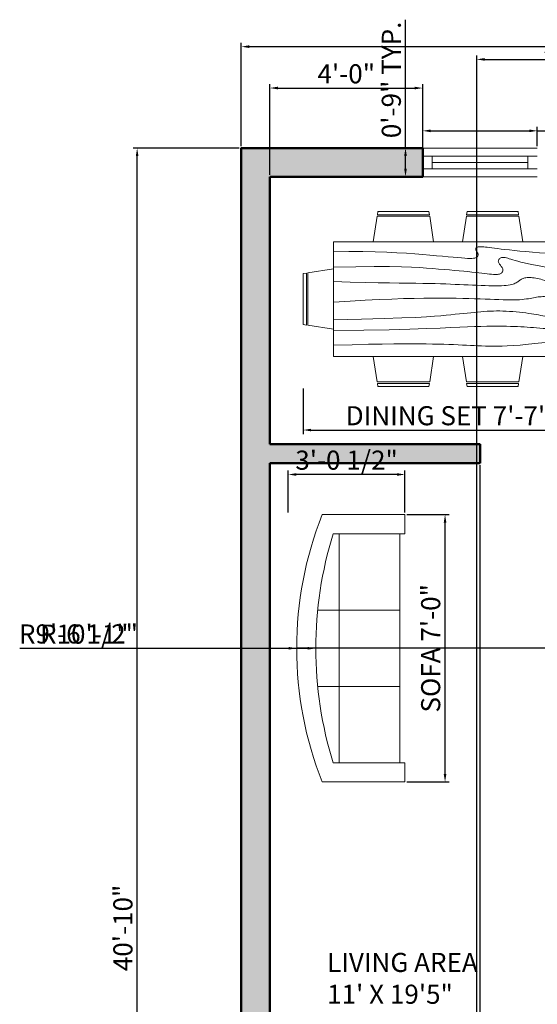
# Model space of a CAD drawing. Units: inches. Extents: x 2247 to 2697, y 1573 to 2133.
# Tile 2 of 4: x 2247 to 2409, y 1823 to 2133. Entities that reach past the tile are written whole.
import ezdxf

# ---------------------------------------------------------------- set-up
doc = ezdxf.new("R2010")
doc.units = ezdxf.units.IN
for name, color, linetype, lineweight in [('A-ANNO-DIMS', 2, 'Continuous', 18), ('A-AREA-IDEN', 7, 'Continuous', 25), ('A-FURN', 8, 'Continuous', 18), ('A-GLAZ', 4, 'Continuous', 18), ('A-WALL', 7, 'Continuous', 50)]:
    doc.layers.add(name, color=color, linetype=linetype, lineweight=lineweight)
doc.layers.add('A-WALL-PATT', color=67, linetype='Continuous', lineweight=13, true_color=0x727430)
doc.styles.get("Standard").update_dxf_attribs({"font": 'arial.ttf'})
doc.dimstyles.new('ISO-25', dxfattribs={"dimtxt": 6, "dimasz": 2.5, "dimexe": 1.25, "dimexo": 0.625, "dimtad": 1, "dimlunit": 3, "dimtxsty": 'Standard', "dimcen": 2.5, "dimadec": 0, "dimazin": 0, "dimtfac": 1, "dimtmove": 0, "dimatfit": 3, "dimfxl": 1, "dimarcsym": 0})

# ---------------------------------------------------------------- blocks, each defined once
blk = doc.blocks.new('*D1')
at = {"layer": 'A-ANNO-DIMS', "color": 0, "lineweight": -2, "transparency": 16777216}
for p, q in [((2316.09, 2092.98), (2316.09, 2125.46)), ((2617.09, 2092.98), (2617.09, 2125.46)), ((2318.59, 2124.21), (2614.59, 2124.21))]:
    blk.add_line(p, q, dxfattribs=at)
at = {"layer": 'A-ANNO-DIMS', "color": 0, "transparency": 16777216}
for points in [[(2318.59, 2124.63), (2318.59, 2123.79), (2316.09, 2124.21)], [(2614.59, 2124.63), (2614.59, 2123.79), (2617.09, 2124.21)]]:
    blk.add_solid(points, dxfattribs=at)
at = {"layer": 'Defpoints', "color": 0, "transparency": 16777216}
for p in [(2617.09, 2124.21), (2316.09, 2092.36), (2617.09, 2092.36)]:
    blk.add_point(p, dxfattribs=at)
at = {"layer": 'A-ANNO-DIMS', "color": 0, "transparency": 16777216, "insert": (2466.59, 2127.9), "char_height": 6, "attachment_point": 5}
blk.add_mtext('25\'-1"', dxfattribs=at)
blk = doc.blocks.new('*D3')
at = {"layer": 'A-ANNO-DIMS', "color": 0, "lineweight": -2, "transparency": 16777216}
for p, q in [((2315.47, 2092.36), (2282.14, 2092.36)), ((2283.39, 1604.86), (2283.39, 2089.86)), ((2315.47, 1602.36), (2282.14, 1602.36))]:
    blk.add_line(p, q, dxfattribs=at)
at = {"layer": 'A-ANNO-DIMS', "color": 0, "transparency": 16777216}
for points in [[(2282.98, 2089.86), (2283.81, 2089.86), (2283.39, 2092.36)], [(2282.98, 1604.86), (2283.81, 1604.86), (2283.39, 1602.36)]]:
    blk.add_solid(points, dxfattribs=at)
at = {"layer": 'Defpoints', "color": 0, "transparency": 16777216}
for p in [(2283.39, 2092.36), (2316.09, 2092.36), (2316.09, 1602.36)]:
    blk.add_point(p, dxfattribs=at)
at = {"layer": 'A-ANNO-DIMS', "color": 0, "transparency": 16777216, "insert": (2279.7, 1847.36), "char_height": 6, "attachment_point": 5, "rotation": 90}
blk.add_mtext('40\'-10"', dxfattribs=at)
blk = doc.blocks.new('Sofa - Roundback 7 ft.')
for p, q in [((-12.00002, -32.4421), (-12.00003, -6.5971)), ((11.99997, -32.4421), (11.99998, -6.5971)), ((-36.000027, -34), (-36.000027, -11.4696)), ((35.99998, -34), (35.99998, -11.4696)), ((-35.999844, -13.3819), (35.9998, -13.3819)), ((-36.000027, -32.4421), (35.99998, -32.4421))]:
    blk.add_line(p, q)
for points in [[(-36.000027, -34), (-42.000027, -34), (-42.000027, -8)], [(41.99998, -8), (41.99998, -34), (35.99998, -34)]]:
    blk.add_lwpolyline(points)
for centre, radius, start, end in [((0, -114.25), 114.25, 68.43141, 111.5686), ((-0.00001, -127.1968), 121.1968, 72.72033, 107.2797)]:
    blk.add_arc(centre, radius, start, end)
blk = doc.blocks.new('Dining Set - 36 x 72 in.')
for p, q in [((-22.2343, 26.00059), (-23.4847, 17.99762)), ((-22.2304, 26), (-5.7608, 26)), ((-22, 27.5), (-22.1562, 26.50042)), ((-5.8416, 26.5), (-22.1534, 26.5)), ((-22, 27.5), (-6, 27.5)), ((-5.8437, 26.49966), (-6, 27.5)), ((-4.5152, 17.99762), (-5.7655, 25.99926)), ((5.7657, 26.00059), (4.5153, 17.99762)), ((5.7696, 26), (22.2392, 26)), ((6, 27.5), (5.8438, 26.50042)), ((22.1584, 26.5), (5.8466, 26.5)), ((6, 27.5), (22, 27.5)), ((22.1563, 26.49966), (22, 27.5)), ((23.4848, 17.99762), (22.2345, 25.99926)), ((36, 18), (-36, 18)), ((-36, 18), (-36, -18)), ((36, -18), (36, 18)), ((-44.0006, 8.23428), (-35.9976, 9.48474)), ((44.0006, 8.23428), (35.9976, 9.48474)), ((-45.5, 8), (-44.5004, 8.15617)), ((-45.5, 8), (-45.5, -8)), ((-44.5, -8.15843), (-44.5, 8.15338)), ((-44, 8.23041), (-44, -8.23915)), ((44, 8.23041), (44, -8.23915)), ((44.5, -8.15843), (44.5, 8.15338)), ((45.5, 8), (44.5005, 8.15617)), ((45.5, 8), (45.5, -8)), ((-44.4997, -8.15631), (-45.5, -8)), ((-35.9976, -9.48476), (-43.9993, -8.2345)), ((35.9976, -9.48476), (43.9993, -8.2345)), ((44.4997, -8.15631), (45.5, -8)), ((-36, -18), (36, -18)), ((-22.2343, -26.0006), (-23.4847, -17.99762)), ((-4.5152, -17.99762), (-5.7655, -25.99928)), ((5.7657, -26.0006), (4.5153, -17.99762)), ((23.4848, -17.99762), (22.2345, -25.99928)), ((-22.2304, -26), (-5.7608, -26)), ((-22, -27.5), (-22.1562, -26.50044)), ((-5.8416, -26.5), (-22.1534, -26.5)), ((-22, -27.5), (-6, -27.5)), ((-5.8437, -26.49967), (-6, -27.5)), ((5.7696, -26), (22.2392, -26)), ((6, -27.5), (5.8438, -26.50044)), ((22.1584, -26.5), (5.8466, -26.5)), ((6, -27.5), (22, -27.5)), ((22.1563, -26.49967), (22, -27.5))]:
    blk.add_line(p, q)
for points in [[(-36, 15), (-31.1772, 14.97754), (-26.8079, 14.91406), (-22.8538, 14.81543), (-19.276, 14.6875), (-16.0362, 14.53613), (-13.0957, 14.36718), (-10.4159, 14.18652), (-7.9583, 14), (-5.6904, 13.81315), (-3.6035, 13.63021), (-1.6954, 13.45508), (0.0365, 13.29166), (1.5945, 13.14388), (2.9811, 13.01562), (4.1988, 12.9108), (5.25, 12.83333), (6.1393, 12.78613), (6.8802, 12.76823), (7.4883, 12.77767), (7.9792, 12.8125), (8.3685, 12.87077), (8.6719, 12.95052), (8.9049, 13.0498), (9.0833, 13.16666), (9.2205, 13.29899), (9.3216, 13.44401), (9.3895, 13.59879), (9.4271, 13.76041), (9.4373, 13.92594), (9.4232, 14.09245), (9.3875, 14.257), (9.3333, 14.41666), (9.2638, 14.56917), (9.1836, 14.71484), (9.0975, 14.85465), (9.0104, 14.98958), (8.9272, 15.1206), (8.8529, 15.2487), (8.7922, 15.37483), (8.75, 15.5), (8.7305, 15.62467), (8.7344, 15.74739), (8.7617, 15.86621), (8.8125, 15.97916), (8.8867, 16.08431), (8.9844, 16.17968), (9.1055, 16.26334), (9.25, 16.33333), (9.4189, 16.38802), (9.6172, 16.42708), (9.8506, 16.45052), (10.125, 16.45833), (10.4463, 16.45052), (10.8203, 16.42708), (11.2529, 16.38802), (11.75, 16.33333), (12.3184, 16.26318), (12.9694, 16.17838), (13.7151, 16.07991), (14.5677, 15.96875), (15.5395, 15.84586), (16.6426, 15.71224), (17.8893, 15.56884), (19.2917, 15.41666), (20.859, 15.25667), (22.5879, 15.08984), (24.4721, 14.91715), (26.5052, 14.73958), (28.6809, 14.5581), (30.9929, 14.3737), (33.4347, 14.18733), (36, 14)], [(-36, 10), (-28.9766, 10.14274), (-23.1725, 10.20442), (-18.4241, 10.19775), (-14.5677, 10.13541), (-11.4399, 10.03011), (-8.877, 9.89453), (-6.7154, 9.74137), (-4.7917, 9.58333), (-2.9698, 9.43082), (-1.2246, 9.28515), (0.4415, 9.14534), (2.026, 9.01041), (3.5266, 8.87939), (4.9408, 8.7513), (6.266, 8.62516), (7.5, 8.5), (8.6411, 8.37549), (9.6914, 8.2539), (10.6538, 8.13818), (11.5312, 8.03125), (12.3267, 7.93603), (13.043, 7.85547), (13.6831, 7.79248), (14.25, 7.75), (14.7471, 7.7303), (15.1797, 7.73307), (15.5537, 7.75732), (15.875, 7.80208), (16.1494, 7.86637), (16.3828, 7.94922), (16.5811, 8.04964), (16.75, 8.16666), (16.8944, 8.29915), (17.0143, 8.44531), (17.1089, 8.60319), (17.1771, 8.77083), (17.218, 8.94629), (17.2305, 9.1276), (17.2137, 9.31282), (17.1667, 9.5), (17.0895, 9.6875), (16.987, 9.875), (16.8649, 10.0625), (16.7292, 10.25), (16.5856, 10.4375), (16.4401, 10.625), (16.2985, 10.8125), (16.1667, 11), (16.05, 11.18733), (15.9518, 11.3737), (15.8752, 11.5581), (15.8229, 11.73958), (15.798, 11.91715), (15.8034, 12.08984), (15.842, 12.25667), (15.9167, 12.41666), (16.0295, 12.56836), (16.1784, 12.70833), (16.3605, 12.83268), (16.5729, 12.9375), (16.8127, 13.01888), (17.0768, 13.07291), (17.3625, 13.0957), (17.6667, 13.08333), (17.9894, 13.03312), (18.3418, 12.94726), (18.7382, 12.82918), (19.1927, 12.68229), (19.7195, 12.51001), (20.3327, 12.31575), (21.0465, 12.10294), (21.875, 11.875), (22.8357, 11.63354), (23.959, 11.37304), (25.2786, 11.08618), (26.8282, 10.76562), (28.6414, 10.40405), (30.752, 9.99414), (33.1936, 9.52856), (36, 9)], [(-36, 5.5), (-30.7157, 5.3348), (-26.069, 5.20963), (-21.9946, 5.11767), (-18.4271, 5.05208), (-15.3009, 5.00602), (-12.5508, 4.97265), (-10.1112, 4.94515), (-7.9167, 4.91666), (-5.909, 4.88167), (-4.0586, 4.83984), (-2.3429, 4.79215), (-0.7396, 4.73958), (0.7739, 4.6831), (2.22, 4.6237), (3.6213, 4.56233), (5, 4.5), (6.373, 4.43782), (7.7344, 4.3776), (9.0723, 4.32129), (10.375, 4.27083), (11.6309, 4.22819), (12.8281, 4.19531), (13.9551, 4.17415), (15, 4.16666), (15.954, 4.17448), (16.819, 4.19791), (17.6001, 4.23698), (18.3021, 4.29166), (18.9299, 4.36198), (19.4883, 4.44791), (19.9823, 4.54948), (20.4167, 4.66666), (20.7969, 4.79899), (21.1302, 4.94401), (21.4245, 5.09879), (21.6875, 5.26041), (21.9271, 5.42594), (22.1511, 5.59245), (22.3672, 5.757), (22.5834, 5.91666), (22.8065, 6.06868), (23.0404, 6.21093), (23.2879, 6.34147), (23.5521, 6.45833), (23.8358, 6.55957), (24.142, 6.64323), (24.4735, 6.70735), (24.8334, 6.75), (25.2235, 6.76969), (25.642, 6.76692), (26.0858, 6.74267), (26.5521, 6.69791), (27.0379, 6.63362), (27.5404, 6.55078), (28.0565, 6.45036), (28.5834, 6.33333), (29.1242, 6.19987), (29.7071, 6.04687), (30.3661, 5.87044), (31.1354, 5.66666), (32.0493, 5.43164), (33.142, 5.16146), (34.4475, 4.85221), (36, 4.5)], [(-36, -1), (-30.7915, -0.6591), (-26.0195, -0.38216), (-21.6519, -0.16284), (-17.6563, 0.00521), (-14.0005, 0.12833), (-10.6523, 0.21289), (-7.5796, 0.26522), (-4.75, 0.29166), (-2.134, 0.29793), (0.2878, 0.28711), (2.5317, 0.26163), (4.6146, 0.22396), (6.5529, 0.17651), (8.3633, 0.12174), (10.0623, 0.06209), (11.6667, 0), (13.1899, -0.06201), (14.6341, -0.1211), (15.9982, -0.17432), (17.2813, -0.21875), (18.4823, -0.25147), (19.6003, -0.26953), (20.6343, -0.27002), (21.5834, -0.25), (22.4481, -0.20768), (23.2357, -0.14584), (23.9549, -0.06836), (24.6146, 0.02083), (25.2235, 0.11784), (25.7904, 0.21875), (26.3241, 0.31966), (26.8334, 0.41666), (27.3265, 0.50618), (27.8099, 0.58593), (28.2894, 0.65397), (28.7709, 0.70833), (29.2601, 0.74707), (29.763, 0.76823), (30.2855, 0.76985), (30.8334, 0.75), (31.4088, 0.70784), (31.9994, 0.64713), (32.589, 0.57275), (33.1615, 0.48958), (33.7008, 0.4025), (34.1908, 0.3164), (34.6153, 0.23616), (34.9584, 0.16666), (35.2099, 0.11165), (35.3848, 0.07031), (35.504, 0.04069), (35.5886, 0.02083), (35.6594, 0.00879), (35.7377, 0.0026), (35.8442, 0.00032), (36, 0)], [(-36, -6.5), (-27.1843, -6.31267), (-20.084, -6.1263), (-14.469, -5.9419), (-10.1094, -5.76042), (-6.7752, -5.58285), (-4.2363, -5.41016), (-2.2629, -5.24333), (-0.625, -5.08334), (0.8708, -4.93099), (2.2715, -4.78646), (3.5872, -4.64974), (4.8281, -4.52084), (6.0046, -4.39974), (7.127, -4.28646), (8.2053, -4.18099), (9.25, -4.08334), (10.2705, -3.99382), (11.2734, -3.91407), (12.2647, -3.84603), (13.25, -3.79167), (14.2354, -3.75293), (15.2266, -3.73177), (16.2295, -3.73015), (17.25, -3.75), (18.2912, -3.79248), (19.3451, -3.85547), (20.4009, -3.93604), (21.4479, -4.03125), (22.4754, -4.13819), (23.4727, -4.25391), (24.4289, -4.37549), (25.3334, -4.5), (26.1785, -4.62492), (26.9694, -4.74935), (27.7145, -4.87281), (28.4219, -4.99479), (29.1, -5.11483), (29.7572, -5.23242), (30.4016, -5.34709), (31.0417, -5.45834), (31.6837, -5.56437), (32.3262, -5.65821), (32.9658, -5.73153), (33.599, -5.77604), (34.2224, -5.78345), (34.8327, -5.74545), (35.4264, -5.65373), (36, -5.5)], [(-36, -10), (-26.4022, -9.81299), (-18.4675, -9.62891), (-11.9839, -9.45069), (-6.7396, -9.28125), (-2.5226, -9.12354), (0.8789, -8.98047), (3.6769, -8.85498), (6.0833, -8.75), (8.2767, -8.66765), (10.3021, -8.60677), (12.1712, -8.56543), (13.8958, -8.54167), (15.4876, -8.53353), (16.9583, -8.53907), (18.3197, -8.55632), (19.5834, -8.58334), (20.7616, -8.61841), (21.8685, -8.66081), (22.9188, -8.71004), (23.9271, -8.76563), (24.9081, -8.82707), (25.8763, -8.89388), (26.8465, -8.96558), (27.8334, -9.04167), (28.8474, -9.12118), (29.8828, -9.20117), (30.93, -9.27824), (31.9792, -9.34896), (33.0205, -9.40991), (34.0443, -9.45768), (35.0407, -9.48885), (36, -9.5)], [(-36, -14.5), (-30.0881, -14.33513), (-25.0332, -14.21224), (-20.7312, -14.12647), (-17.0781, -14.07292), (-13.97, -14.04671), (-11.3027, -14.04297), (-8.9724, -14.05681), (-6.875, -14.08334), (-4.9224, -14.11833), (-3.0905, -14.16016), (-1.3709, -14.20785), (0.2448, -14.26042), (1.7647, -14.3169), (3.1973, -14.3763), (4.5507, -14.43767), (5.8333, -14.5), (7.0554, -14.5621), (8.235, -14.62175), (9.3922, -14.67652), (10.5469, -14.72396), (11.7192, -14.76164), (12.929, -14.78711), (14.1965, -14.79794), (15.5417, -14.79167), (16.9933, -14.76424), (18.6152, -14.70508), (20.4804, -14.60197), (22.6615, -14.44271), (25.2312, -14.21509), (28.2624, -13.9069), (31.8277, -13.50594), (36, -13)]]:
    blk.add_lwpolyline(points)
blk = doc.blocks.new('WIN-36IN')
for p, q in [((0, 9), (36, 9)), ((0, 6.5), (36, 6.5)), ((3, 2.5), (3, 6.5)), ((33, 2.5), (33, 6.5)), ((3, 4.5), (33, 4.5)), ((0, 2.5), (36, 2.5)), ((0, 0), (36, 0))]:
    blk.add_line(p, q)
blk = doc.blocks.new('*D13')
at = {"layer": 'A-ANNO-DIMS', "color": 0, "lineweight": -2, "transparency": 16777216}
for p, q in [((2373.09, 2092.98), (2373.09, 2099.01)), ((2375.59, 2097.76), (2406.59, 2097.76)), ((2409.09, 2092.98), (2409.09, 2099.01)), ((2409.09, 2097.76), (2488.77, 2097.76))]:
    blk.add_line(p, q, dxfattribs=at)
at = {"layer": 'A-ANNO-DIMS', "color": 0, "transparency": 16777216}
for points in [[(2375.59, 2098.18), (2375.59, 2097.34), (2373.09, 2097.76)], [(2406.59, 2098.18), (2406.59, 2097.34), (2409.09, 2097.76)]]:
    blk.add_solid(points, dxfattribs=at)
at = {"layer": 'Defpoints', "color": 0, "transparency": 16777216}
for p in [(2409.09, 2097.76), (2373.09, 2092.36), (2409.09, 2092.36)]:
    blk.add_point(p, dxfattribs=at)
at = {"layer": 'A-ANNO-DIMS', "color": 0, "transparency": 16777216, "insert": (2450.18, 2101.49), "char_height": 6, "attachment_point": 5}
blk.add_mtext('WINDOW 3\'-0" TYP.', dxfattribs=at)
blk = doc.blocks.new('*D14')
at = {"layer": 'A-ANNO-DIMS', "color": 0, "lineweight": -2, "transparency": 16777216}
for p, q in [((2367.69, 2092.36), (2367.69, 2132.68)), ((2372.47, 2092.36), (2366.44, 2092.36)), ((2367.69, 2085.86), (2367.69, 2089.86)), ((2372.47, 2083.36), (2366.44, 2083.36))]:
    blk.add_line(p, q, dxfattribs=at)
at = {"layer": 'A-ANNO-DIMS', "color": 0, "transparency": 16777216}
for points in [[(2367.28, 2089.86), (2368.11, 2089.86), (2367.69, 2092.36)], [(2367.28, 2085.86), (2368.11, 2085.86), (2367.69, 2083.36)]]:
    blk.add_solid(points, dxfattribs=at)
at = {"layer": 'Defpoints', "color": 0, "transparency": 16777216}
for p in [(2367.69, 2092.36), (2373.09, 2092.36), (2373.09, 2083.36)]:
    blk.add_point(p, dxfattribs=at)
at = {"layer": 'A-ANNO-DIMS', "color": 0, "transparency": 16777216, "insert": (2364.01, 2113.77), "char_height": 6, "attachment_point": 5, "rotation": 90}
blk.add_mtext('0\'-9" TYP.', dxfattribs=at)
blk = doc.blocks.new('*D19')
at = {"layer": 'A-ANNO-DIMS', "color": 0, "lineweight": -2, "transparency": 16777216}
for p, q in [((2368.14, 1977.2), (2381.36, 1977.2)), ((2380.11, 1895.7), (2380.11, 1974.7)), ((2368.14, 1893.2), (2381.36, 1893.2))]:
    blk.add_line(p, q, dxfattribs=at)
at = {"layer": 'A-ANNO-DIMS', "color": 0, "transparency": 16777216}
for points in [[(2379.7, 1974.7), (2380.53, 1974.7), (2380.11, 1977.2)], [(2379.7, 1895.7), (2380.53, 1895.7), (2380.11, 1893.2)]]:
    blk.add_solid(points, dxfattribs=at)
at = {"layer": 'Defpoints', "color": 0, "transparency": 16777216}
for p in [(2367.51, 1977.2), (2380.11, 1977.2), (2367.51, 1893.2)]:
    blk.add_point(p, dxfattribs=at)
at = {"layer": 'A-ANNO-DIMS', "color": 0, "transparency": 16777216, "insert": (2376.38, 1935.2), "char_height": 6, "attachment_point": 5, "rotation": 90}
blk.add_mtext('SOFA 7\'-0"', dxfattribs=at)
blk = doc.blocks.new('*D20')
at = {"layer": 'A-ANNO-DIMS', "color": 0, "lineweight": -2, "transparency": 16777216}
for p, q in [((2330.85, 1977.83), (2330.85, 1991.05)), ((2365.01, 1989.8), (2333.35, 1989.8)), ((2367.51, 1977.83), (2367.51, 1991.05))]:
    blk.add_line(p, q, dxfattribs=at)
at = {"layer": 'A-ANNO-DIMS', "color": 0, "transparency": 16777216}
for points in [[(2333.35, 1990.22), (2333.35, 1989.39), (2330.85, 1989.8)], [(2365.01, 1990.22), (2365.01, 1989.39), (2367.51, 1989.8)]]:
    blk.add_solid(points, dxfattribs=at)
at = {"layer": 'Defpoints', "color": 0, "transparency": 16777216}
for p in [(2330.85, 1989.8), (2330.85, 1977.2), (2367.51, 1977.2)]:
    blk.add_point(p, dxfattribs=at)
at = {"layer": 'A-ANNO-DIMS', "color": 0, "transparency": 16777216, "insert": (2349.18, 1993.53), "char_height": 6, "attachment_point": 5}
blk.add_mtext('3\'-0 1/2"', dxfattribs=at)
blk = doc.blocks.new('*D21')
at = {"layer": 'A-ANNO-DIMS', "color": 0, "lineweight": -2, "transparency": 16777216}
for p, q in [((2335.55, 2016.79), (2335.55, 2002.52)), ((2426.55, 2016.79), (2426.55, 2002.52)), ((2338.05, 2003.77), (2424.05, 2003.77))]:
    blk.add_line(p, q, dxfattribs=at)
at = {"layer": 'A-ANNO-DIMS', "color": 0, "transparency": 16777216}
for points in [[(2338.05, 2004.18), (2338.05, 2003.35), (2335.55, 2003.77)], [(2424.05, 2004.18), (2424.05, 2003.35), (2426.55, 2003.77)]]:
    blk.add_solid(points, dxfattribs=at)
at = {"layer": 'Defpoints', "color": 0, "transparency": 16777216}
for p in [(2335.55, 2017.42), (2426.55, 2017.42), (2426.55, 2003.77)]:
    blk.add_point(p, dxfattribs=at)
at = {"layer": 'A-ANNO-DIMS', "color": 0, "transparency": 16777216, "insert": (2381.05, 2007.49), "char_height": 6, "attachment_point": 5}
blk.add_mtext('DINING SET 7\'-7"', dxfattribs=at)
blk = doc.blocks.new('*D23')
at = {"layer": 'A-ANNO-DIMS', "color": 0, "lineweight": -2, "transparency": 16777216}
for p, q in [((2325.09, 2083.98), (2325.09, 2112.46)), ((2327.59, 2111.21), (2370.59, 2111.21)), ((2373.09, 2083.98), (2373.09, 2112.46))]:
    blk.add_line(p, q, dxfattribs=at)
at = {"layer": 'A-ANNO-DIMS', "color": 0, "transparency": 16777216}
for points in [[(2327.59, 2111.63), (2327.59, 2110.79), (2325.09, 2111.21)], [(2370.59, 2111.63), (2370.59, 2110.79), (2373.09, 2111.21)]]:
    blk.add_solid(points, dxfattribs=at)
at = {"layer": 'Defpoints', "color": 0, "transparency": 16777216}
for p in [(2373.09, 2111.21), (2325.09, 2083.36), (2373.09, 2083.36)]:
    blk.add_point(p, dxfattribs=at)
at = {"layer": 'A-ANNO-DIMS', "color": 0, "transparency": 16777216, "insert": (2349.09, 2114.9), "char_height": 6, "attachment_point": 5}
blk.add_mtext('4\'-0"', dxfattribs=at)
blk = doc.blocks.new('*D38')
at = {"layer": 'A-ANNO-DIMS', "color": 0, "lineweight": -2, "transparency": 16777216}
for p, q in [((2390.09, 1693.98), (2390.09, 2121.46)), ((2392.59, 2120.21), (2447.59, 2120.21)), ((2450.09, 1693.98), (2450.09, 2121.46))]:
    blk.add_line(p, q, dxfattribs=at)
at = {"layer": 'A-ANNO-DIMS', "color": 0, "transparency": 16777216}
for points in [[(2392.59, 2120.63), (2392.59, 2119.79), (2390.09, 2120.21)], [(2447.59, 2120.63), (2447.59, 2119.79), (2450.09, 2120.21)]]:
    blk.add_solid(points, dxfattribs=at)
at = {"layer": 'Defpoints', "color": 0, "transparency": 16777216}
for p in [(2450.09, 2120.21), (2390.09, 1693.36), (2450.09, 1693.36)]:
    blk.add_point(p, dxfattribs=at)
at = {"layer": 'A-ANNO-DIMS', "color": 0, "transparency": 16777216, "insert": (2420.09, 2123.9), "char_height": 6, "attachment_point": 5}
blk.add_mtext('5\'-0"', dxfattribs=at)
blk = doc.blocks.new('*D39')
at = {"layer": 'A-ANNO-DIMS', "color": 0, "lineweight": -2, "transparency": 16777216}
for p, q in [((2325.09, 1992.73), (2325.09, 1573.26)), ((2391.09, 1992.73), (2391.09, 1573.26)), ((2327.59, 1574.51), (2388.59, 1574.51))]:
    blk.add_line(p, q, dxfattribs=at)
at = {"layer": 'A-ANNO-DIMS', "color": 0, "transparency": 16777216}
for points in [[(2327.59, 1574.93), (2327.59, 1574.09), (2325.09, 1574.51)], [(2388.59, 1574.93), (2388.59, 1574.09), (2391.09, 1574.51)]]:
    blk.add_solid(points, dxfattribs=at)
at = {"layer": 'Defpoints', "color": 0, "transparency": 16777216}
for p in [(2325.09, 1993.36), (2391.09, 1993.36), (2391.09, 1574.51)]:
    blk.add_point(p, dxfattribs=at)
at = {"layer": 'A-ANNO-DIMS', "color": 0, "transparency": 16777216, "insert": (2358.09, 1578.2), "char_height": 6, "attachment_point": 5}
blk.add_mtext('5\'-6"', dxfattribs=at)
blk = doc.blocks.new('*D40')
at = {"layer": 'A-ANNO-DIMS', "color": 0, "lineweight": -2, "transparency": 16777216}
for p, q in [((2391.09, 1992.73), (2391.09, 1573.26)), ((2439.09, 1992.73), (2439.09, 1573.26)), ((2393.59, 1574.51), (2436.59, 1574.51))]:
    blk.add_line(p, q, dxfattribs=at)
at = {"layer": 'A-ANNO-DIMS', "color": 0, "transparency": 16777216}
for points in [[(2393.59, 1574.93), (2393.59, 1574.09), (2391.09, 1574.51)], [(2436.59, 1574.93), (2436.59, 1574.09), (2439.09, 1574.51)]]:
    blk.add_solid(points, dxfattribs=at)
at = {"layer": 'Defpoints', "color": 0, "transparency": 16777216}
for p in [(2391.09, 1993.36), (2439.09, 1993.36), (2439.09, 1574.51)]:
    blk.add_point(p, dxfattribs=at)
at = {"layer": 'A-ANNO-DIMS', "color": 0, "transparency": 16777216, "insert": (2415.09, 1578.2), "char_height": 6, "attachment_point": 5}
blk.add_mtext('4\'-0"', dxfattribs=at)
blk = doc.blocks.new('*D49')
at = {"layer": 'A-ANNO-DIMS', "color": 0, "lineweight": -2, "transparency": 16777216}
for p, q in [((2252.99, 1935.2), (2337.01, 1935.2)), ((2460.71, 1935.2), (2339.51, 1935.2))]:
    blk.add_line(p, q, dxfattribs=at)
at = {"layer": 'A-ANNO-DIMS', "color": 0, "transparency": 16777216}
blk.add_solid([(2337.01, 1935.62), (2337.01, 1934.79), (2339.51, 1935.2)], dxfattribs=at)
at = {"layer": 'Defpoints', "color": 0, "transparency": 16777216}
for p in [(2339.51, 1935.2), (2460.71, 1935.2)]:
    blk.add_point(p, dxfattribs=at)
at = {"layer": 'A-ANNO-DIMS', "color": 0, "transparency": 16777216, "insert": (2266.79, 1938.89), "char_height": 6, "attachment_point": 5}
blk.add_mtext('R10\'-1"', dxfattribs=at)
blk = doc.blocks.new('*D50')
at = {"layer": 'A-ANNO-DIMS', "color": 0, "lineweight": -2, "transparency": 16777216}
for p, q in [((2246.5, 1935.2), (2331.01, 1935.2)), ((2447.76, 1935.2), (2333.51, 1935.2))]:
    blk.add_line(p, q, dxfattribs=at)
at = {"layer": 'A-ANNO-DIMS', "color": 0, "transparency": 16777216}
blk.add_solid([(2331.01, 1935.62), (2331.01, 1934.79), (2333.51, 1935.2)], dxfattribs=at)
at = {"layer": 'Defpoints', "color": 0, "transparency": 16777216}
for p in [(2333.51, 1935.2), (2447.76, 1935.2)]:
    blk.add_point(p, dxfattribs=at)
at = {"layer": 'A-ANNO-DIMS', "color": 0, "transparency": 16777216, "insert": (2264.96, 1938.93), "char_height": 6, "attachment_point": 5}
blk.add_mtext('R9\'-6 1/2"', dxfattribs=at)

msp = doc.modelspace()

# ---------------------------------------------------------------- hatches: boundary and pattern name
at = {"layer": 'A-WALL-PATT'}
h = msp.add_hatch(color=256, dxfattribs=at)
h.dxf.hatch_style = 1
h.paths.add_polyline_path([(2325.094, 1993.36), (2391.094, 1993.36), (2391.094, 1999.36), (2325.094, 1999.36), (2325.094, 2083.36), (2373.094, 2083.36), (2373.094, 2092.36), (2316.094, 2092.36), (2316.094, 1687.36), (2337.094, 1687.36), (2337.094, 1693.36), (2325.094, 1693.36), (2325.094, 1753.36), (2379.094, 1753.36), (2379.094, 1759.36), (2325.094, 1759.36)])

# ---------------------------------------------------------------- linework, layer by layer
at = {"layer": 'A-WALL'}
for p, q in [((2373.094, 2083.36), (2373.094, 2092.36)), ((2325.094, 2083.36), (2373.094, 2083.36)), ((2325.094, 1999.36), (2325.094, 2083.36)), ((2325.094, 1999.36), (2391.094, 1999.36)), ((2391.094, 1993.36), (2391.094, 1999.36)), ((2325.094, 1993.36), (2391.094, 1993.36)), ((2325.094, 1759.36), (2325.094, 1993.36))]:
    msp.add_line(p, q, dxfattribs=at)
msp.add_lwpolyline([(2316.094, 1687.36), (2316.094, 2092.36), (2373.094, 2092.36)], dxfattribs=at)

# ---------------------------------------------------------------- block references
at = {"layer": 'A-FURN'}
msp.add_blockref('Dining Set - 36 x 72 in.', (2381.053, 2044.916), dxfattribs=at)
at = {"layer": 'A-FURN', "rotation": 90}
msp.add_blockref('Sofa - Roundback 7 ft.', (2333.513, 1935.202), dxfattribs=at)
at = {"layer": 'A-GLAZ'}
msp.add_blockref('WIN-36IN', (2373.094, 2083.36), dxfattribs=at)

# ---------------------------------------------------------------- texts
at = {"layer": 'A-AREA-IDEN', "insert": (2343.069, 1839.519), "char_height": 6, "attachment_point": 1}
msp.add_mtext_dynamic_manual_height_columns('{\\fArial|b1|i0|c0|p34;LIVING AREA \\P11\' X 19\'5"}', width=77.17846, gutter_width=12.5, heights=[0], dxfattribs=at)

# ---------------------------------------------------------------- dimensions: what is measured, and where the dimension line sits
at = {"layer": 'A-ANNO-DIMS'}
for base, p1, p2, override, picture, middle in [((2617.094, 2124.211), (2316.094, 2092.36), (2617.094, 2092.36), {"dimclrd": 0, "dimclre": 0, "dimclrt": 0}, '*D1', (2466.594, 2127.899)), ((2450.094, 2120.21), (2390.094, 1693.36), (2450.094, 1693.36), {"dimdec": 1, "dimlfac": 1, "dimrnd": 0, "dimzin": 1, "dimdsep": 46, "dimlunit": 4, "dimfrac": 2}, '*D38', (2420.094, 2123.898)), ((2373.094, 2111.21), (2325.094, 2083.36), (2373.094, 2083.36), {"dimdec": 1, "dimlfac": 1, "dimrnd": 0, "dimzin": 1, "dimdsep": 46, "dimlunit": 4, "dimfrac": 2}, '*D23', (2349.094, 2114.898)), ((2391.094, 1574.51), (2325.094, 1993.36), (2391.094, 1993.36), {"dimdec": 1, "dimlfac": 1, "dimrnd": 0, "dimzin": 1, "dimdsep": 46, "dimlunit": 4, "dimfrac": 2}, '*D39', (2358.094, 1578.198)), ((2439.094, 1574.51), (2391.094, 1993.36), (2439.094, 1993.36), {"dimdec": 1, "dimlfac": 1, "dimrnd": 0, "dimzin": 1, "dimdsep": 46, "dimlunit": 4, "dimfrac": 2}, '*D40', (2415.094, 1578.198))]:
    dim = msp.add_linear_dim(base=base, p1=p1, p2=p2, dimstyle='ISO-25', override=override, dxfattribs=at)
    dim.commit()
    dim.dimension.update_dxf_attribs({"geometry": picture, "text_midpoint": middle})
for base, p1, p2, text, picture, middle in [((2367.694, 2092.36), (2373.094, 2083.36), (2373.094, 2092.36), '<> TYP.', '*D14', (2364.006, 2113.771)), ((2380.113, 1977.202), (2367.513, 1893.202), (2367.513, 1977.202), 'SOFA <>', '*D19', (2376.384, 1935.202))]:
    dim = msp.add_linear_dim(base=base, p1=p1, p2=p2, angle=90, text=text, dimstyle='ISO-25', override={"dimdec": 1, "dimlfac": 1, "dimrnd": 0, "dimzin": 1, "dimdsep": 46, "dimlunit": 4, "dimfrac": 2}, dxfattribs=at)
    dim.commit()
    dim.dimension.update_dxf_attribs({"geometry": picture, "text_midpoint": middle})
for base, p1, p2, text, picture, middle in [((2409.094, 2097.76), (2373.094, 2092.36), (2409.094, 2092.36), 'WINDOW <> TYP.', '*D13', (2450.182, 2101.491)), ((2426.553, 2003.766), (2335.553, 2017.416), (2426.553, 2017.416), 'DINING SET <>', '*D21', (2381.053, 2007.493))]:
    dim = msp.add_linear_dim(base=base, p1=p1, p2=p2, text=text, dimstyle='ISO-25', override={"dimdec": 1, "dimlfac": 1, "dimrnd": 0, "dimzin": 1, "dimdsep": 46, "dimlunit": 4, "dimfrac": 2}, dxfattribs=at)
    dim.commit()
    dim.dimension.update_dxf_attribs({"geometry": picture, "text_midpoint": middle})
for base, p1, p2, angle, override, picture, middle in [((2283.393, 2092.36), (2316.094, 1602.36), (2316.094, 2092.36), 90, {"dimclrd": 0, "dimclre": 0, "dimclrt": 0}, '*D3', (2279.704, 1847.36)), ((2330.846, 1989.802), (2367.513, 1977.202), (2330.846, 1977.202), 180, {"dimdec": 1, "dimlfac": 1, "dimrnd": 0, "dimzin": 1, "dimdsep": 46, "dimlunit": 4, "dimfrac": 2}, '*D20', (2349.18, 1993.531))]:
    dim = msp.add_linear_dim(base=base, p1=p1, p2=p2, angle=angle, dimstyle='ISO-25', override=override, dxfattribs=at)
    dim.commit()
    dim.dimension.update_dxf_attribs({"geometry": picture, "text_midpoint": middle})
for center, mpoint, picture, middle in [((2447.762936, 1935.202052), (2333.512936, 1935.202), '*D50', (2264.962936, 1935.202)), ((2460.71, 1935.202), (2339.513, 1935.202), '*D49', (2266.795, 1935.202))]:
    dim = msp.add_radius_dim(center=center, mpoint=mpoint, dimstyle='ISO-25', override={"dimdec": 1, "dimlfac": 1, "dimrnd": 0, "dimzin": 1, "dimdsep": 46, "dimlunit": 4, "dimfrac": 2}, dxfattribs=at)
    dim.commit()
    dim.dimension.update_dxf_attribs({"geometry": picture, "text_midpoint": middle, "dimtype": 164})

doc.saveas('drawing.dxf')
